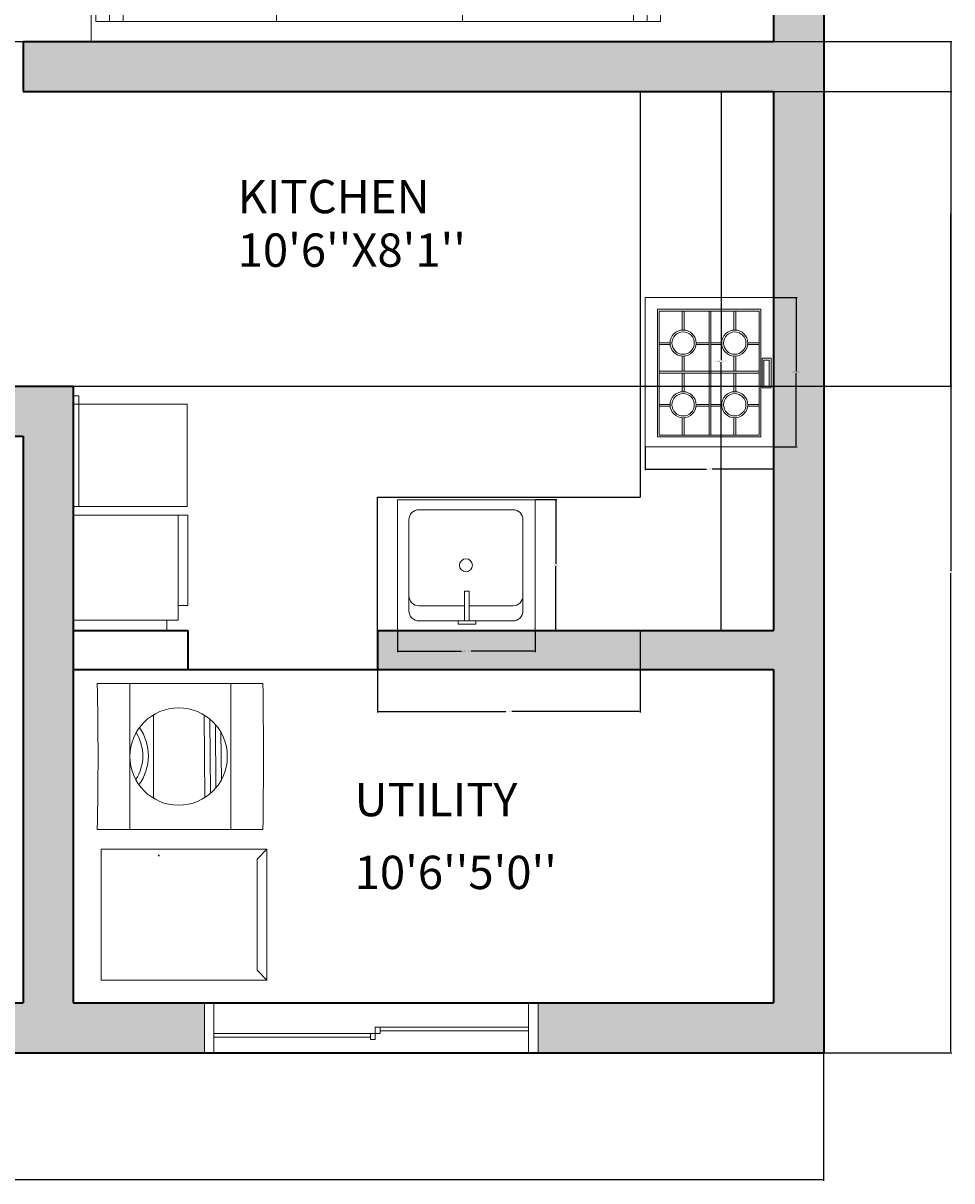
# Model space of a CAD drawing. Units: inches. Extents: x 1789 to 2841, y 3180 to 3702.
# Tile 4 of 14: x 2181 to 2348, y 3180 to 3388. Entities that reach past the tile are written whole.
import ezdxf

# ---------------------------------------------------------------- set-up
doc = ezdxf.new("R2010")
doc.units = ezdxf.units.IN
doc.header["$MEASUREMENT"] = 0
for name, color, linetype, lineweight in [('A-ANNO-DIMS', 2, 'Continuous', 18), ('A-AREA-IDEN', 7, 'Continuous', 18), ('A-EQPM', 8, 'Continuous', 18), ('A-FLOR-CASE', 34, 'Continuous', 25), ('A-FLOR-FIXT', 9, 'Continuous', 18), ('A-WALL', 40, 'Continuous', 35), ('A-WALL-PATT', 252, 'Continuous', 13), ('FURNITURE', 34, 'Continuous', 18), ('WINDOWS', 130, 'Continuous', 18)]:
    doc.layers.add(name, color=color, linetype=linetype, lineweight=lineweight)
doc.styles.get("Standard").update_dxf_attribs({"font": 'arial.ttf'})
doc.dimstyles.get("Standard").update_dxf_attribs({"dimtxt": 0.18, "dimasz": 0.18, "dimexe": 0.18, "dimexo": 0.0625, "dimgap": 0.09, "dimtad": 0, "dimtih": 1, "dimtoh": 1, "dimdec": 0, "dimzin": 0, "dimdsep": 46, "dimlunit": 3, "dimtxsty": 'Standard', "dimcen": 0.09, "dimadec": 0, "dimazin": 0, "dimtfac": 1, "dimtdec": 0, "dimtofl": 0, "dimtmove": 0, "dimatfit": 3, "dimfxl": 1, "dimtolj": 1, "dimtzin": 0, "dimarcsym": 0})

# ---------------------------------------------------------------- blocks, each defined once
blk = doc.blocks.new('HYJ')
for p, q in [((2236.02, 3650.77), (2262.74, 3650.77)), ((2236.02, 3650.11), (2262.74, 3650.11)), ((2206.12, 3649.67), (2234.3, 3649.67)), ((2206.12, 3649), (2234.3, 3649))]:
    blk.add_line(p, q)
for points in [[(2204.43, 3646.16), (2264.43, 3646.16), (2264.43, 3655.16), (2204.43, 3655.16)], [(2204.43, 3655.16), (2206.12, 3655.16), (2206.12, 3646.16), (2204.43, 3646.16)], [(2264.43, 3655.16), (2262.74, 3655.16), (2262.74, 3646.16), (2264.43, 3646.16)], [(2235.16, 3650.77), (2236.02, 3650.77), (2236.02, 3649.67), (2235.16, 3649.67)], [(2234.3, 3649.67), (2235.16, 3649.67), (2235.16, 3648.56), (2234.3, 3648.56)]]:
    blk.add_lwpolyline(points, close=True)
blk = doc.blocks.new('WASH')
for p, q in [((2194.57, 3269.63), (2224.37, 3269.63)), ((2200.44, 3243.35), (2200.44, 3269.63)), ((2218.58, 3269.63), (2218.58, 3243.35)), ((2204.7, 3264.01), (2204.68, 3248.99)), ((2213.79, 3263.95), (2213.93, 3249.12)), ((2214.8, 3263.23), (2214.92, 3249.86)), ((2215.81, 3262.24), (2215.91, 3250.86)), ((2216.82, 3260.81), (2216.9, 3252.31)), ((2194.57, 3243.35), (2224.37, 3243.35)), ((2225.07, 3239.8), (2223.31, 3238.03)), ((2223.31, 3218.04), (2223.31, 3238.03)), ((2225.07, 3216.27), (2223.31, 3218.04))]:
    blk.add_line(p, q)
blk.add_lwpolyline([(2195.28, 3239.8), (2225.07, 3239.8), (2225.07, 3216.27), (2195.28, 3216.27)], close=True)
blk.add_circle((2209.2, 3256.49), 8.76)
for centre, radius, start, end in [((1539.89, 3256.49), 654.81, 358.85012, 1.14988), ((1226.25, 3256.49), 998.2, 359.24572, 0.75428), ((2194.95, 3256.62), 7.81, 326.7676, 32.1994), ((2194.95, 3256.62), 8.81, 323.7828, 35.1842)]:
    blk.add_arc(centre, radius, start, end)
blk = doc.blocks.new('SINK')
for points in [[(2247.56, 3305.33), (2275.07, 3305.33), (2275.07, 3279.16), (2247.56, 3279.16)], [(2260.91, 3287.01), (2261.87, 3287.01), (2261.87, 3281.09), (2260.91, 3281.09)], [(2259.67, 3281.09), (2263.21, 3281.09), (2263.21, 3280.41), (2259.67, 3280.41)]]:
    blk.add_lwpolyline(points, close=True)
blk.add_lwpolyline([(2251.84, 3281.09), (2270.63, 3281.09, 0.414214), (2272.63, 3283.09), (2272.63, 3301.33, 0.414214), (2270.63, 3303.33), (2251.84, 3303.33, 0.414214), (2249.84, 3301.33), (2249.84, 3283.09, 0.414214)], format="xyb", close=True)
for points in [[(2249.84, 3301.33), (2249.84, 3286.11, 0.414214), (2251.84, 3284.11), (2260.91, 3284.11)], [(2261.87, 3284.11), (2270.63, 3284.11, 0.414214), (2272.63, 3286.11), (2272.63, 3301.33)]]:
    blk.add_lwpolyline(points, format="xyb")
blk.add_circle((2261.24, 3292.21), 1.3)
blk = doc.blocks.new('STOVE')
for p, q in [((2291.13, 3337.23), (2291.13, 3342.37)), ((2291.63, 3337.23), (2291.63, 3342.37)), ((2298.52, 3342.42), (2298.52, 3308.4)), ((2299.02, 3342.42), (2299.02, 3308.4)), ((2305.31, 3337.23), (2305.31, 3342.37)), ((2305.81, 3337.23), (2305.81, 3342.37)), ((2287.79, 3333.73), (2284.84, 3333.73)), ((2287.81, 3333.23), (2284.84, 3333.23)), ((2294.92, 3333.23), (2298.52, 3333.23)), ((2294.94, 3333.73), (2298.52, 3333.73)), ((2301.97, 3333.73), (2299.02, 3333.73)), ((2301.99, 3333.23), (2299.02, 3333.23)), ((2309.1, 3333.23), (2312.22, 3333.23)), ((2309.12, 3333.73), (2312.22, 3333.73)), ((2291.13, 3330.09), (2291.13, 3325.91)), ((2291.63, 3330.09), (2291.63, 3325.91)), ((2305.31, 3330.09), (2305.31, 3325.91)), ((2305.81, 3330.09), (2305.81, 3325.91)), ((2284.82, 3325.91), (2312.22, 3325.91)), ((2284.82, 3325.41), (2312.22, 3325.41)), ((2291.15, 3320.29), (2291.15, 3325.43)), ((2291.65, 3320.29), (2291.65, 3325.43)), ((2305.31, 3320.29), (2305.31, 3325.43)), ((2305.31, 3325.41), (2305.31, 3325.34)), ((2305.81, 3320.29), (2305.81, 3325.43)), ((2305.81, 3325.41), (2305.81, 3325.34)), ((2287.8, 3316.79), (2284.82, 3316.79)), ((2287.83, 3316.29), (2284.82, 3316.29)), ((2294.94, 3316.29), (2298.52, 3316.29)), ((2294.96, 3316.79), (2298.52, 3316.79)), ((2301.97, 3316.79), (2299.02, 3316.79)), ((2301.99, 3316.29), (2299.02, 3316.29)), ((2309.1, 3316.29), (2312.22, 3316.29)), ((2309.12, 3316.79), (2312.22, 3316.79)), ((2291.15, 3313.15), (2291.15, 3308.4)), ((2291.65, 3313.15), (2291.65, 3308.4)), ((2305.31, 3313.15), (2305.31, 3308.4)), ((2305.81, 3313.15), (2305.81, 3308.4))]:
    blk.add_line(p, q)
for points in [[(2280.96, 3346.14), (2316.23, 3346.14), (2316.23, 3305.13), (2280.96, 3305.13)], [(2284.32, 3342.92), (2312.72, 3342.92), (2312.72, 3307.9), (2284.32, 3307.9)], [(2284.82, 3342.42), (2312.22, 3342.42), (2312.22, 3308.4), (2284.82, 3308.4)], [(2313.05, 3329.49), (2315.55, 3329.49), (2315.55, 3321.33), (2313.05, 3321.33)], [(2313.55, 3328.99), (2315.05, 3328.99), (2315.05, 3321.83), (2313.55, 3321.83)]]:
    blk.add_lwpolyline(points, close=True)
for centre, radius in [((2291.37, 3333.66), 3.58), ((2291.37, 3333.66), 3.08), ((2305.55, 3333.66), 3.58), ((2305.55, 3333.66), 3.08), ((2291.38, 3316.72), 3.58), ((2291.38, 3316.72), 3.08), ((2305.55, 3316.72), 3.58), ((2305.55, 3316.72), 3.08)]:
    blk.add_circle(centre, radius)
blk = doc.blocks.new('BYY')
for p, q in [((2191.23, 3321.4), (2190.23, 3321.4)), ((2190.23, 3321.4), (2190.23, 3319.89)), ((2191.23, 3301.51), (2191.23, 3321.4)), ((2209.12, 3299.92), (2210.83, 3299.92)), ((2210.83, 3299.92), (2210.83, 3283.66)), ((2210.83, 3283.66), (2209.12, 3283.66)), ((2190.23, 3279.16), (2190.23, 3281.03)), ((2207.05, 3279.16), (2190.23, 3279.16)), ((2207.05, 3281.03), (2207.05, 3279.16))]:
    blk.add_line(p, q)
for points in [[(2190.23, 3319.89), (2210.75, 3319.89), (2210.75, 3301.51), (2190.23, 3301.51)], [(2190.23, 3281.03), (2209.12, 3281.03), (2209.12, 3299.92), (2190.23, 3299.92)]]:
    blk.add_lwpolyline(points, close=True)
blk = doc.blocks.new('SOFA')
for p, q in [((2185.57, 3479.13), (2185.57, 3482.99)), ((2185.57, 3482.99), (2290.09, 3482.99)), ((2290.09, 3482.99), (2290.09, 3460.33)), ((2159.93, 3439.46), (2194.03, 3439.46)), ((2226.79, 3388.76), (2226.79, 3418.07)), ((2260.29, 3388.76), (2260.29, 3418.07)), ((2310.14, 3409.22), (2310.14, 3394.77))]:
    blk.add_line(p, q)
for points in [[(2168.05, 3468.75), (2193.44, 3468.75), (2193.44, 3479.13), (2168.05, 3479.13)], [(2304.69, 3457.56), (2311.21, 3457.56), (2311.21, 3434.14), (2304.69, 3434.14)], [(2227.7, 3454.8), (2263.24, 3454.8), (2263.24, 3433.45), (2227.7, 3433.45)], [(2168.05, 3410.16), (2193.44, 3410.16), (2193.44, 3385.14), (2168.05, 3385.14)], [(2296.77, 3394.77), (2311.21, 3394.77), (2311.21, 3409.22), (2296.77, 3409.22)]]:
    blk.add_lwpolyline(points, close=True)
for points in [[(2168.05, 3467.86), (2168.05, 3470.06, 0.414214), (2166.05, 3472.06), (2155.57, 3472.06), (2155.57, 3406.2), (2166.05, 3406.2, 0.414214), (2168.05, 3408.2), (2168.05, 3411.06)], [(2308.49, 3457.56), (2308.49, 3460.33), (2286.26, 3460.33, 0.414214), (2285.26, 3459.33), (2285.26, 3455.79, 0.414214), (2286.26, 3454.79), (2304.69, 3454.79)], [(2308.49, 3434.14), (2308.49, 3431.37), (2286.26, 3431.37, -0.414214), (2285.26, 3432.37), (2285.26, 3435.9, -0.414214), (2286.26, 3436.9), (2304.69, 3436.9)], [(2196.77, 3407.83), (2196.77, 3416.07, -0.414214), (2198.77, 3418.07), (2291.47, 3418.07, -0.414214), (2293.47, 3416.07), (2293.47, 3407.83)], [(2293.47, 3393.66, 0.414214), (2291.47, 3395.66), (2198.77, 3395.66, 0.414214), (2196.77, 3393.66)]]:
    blk.add_lwpolyline(points, format="xyb")
for points in [[(2159.93, 3468.75), (2192.03, 3468.75, -0.414214), (2194.03, 3466.75), (2194.03, 3412.16, -0.414214), (2192.03, 3410.16), (2159.93, 3410.16)], [(2284.53, 3460.33), (2311.21, 3460.33), (2311.21, 3431.37), (2284.53, 3431.37, -0.414214), (2282.53, 3433.37), (2282.53, 3458.33, -0.414214)], [(2197.2, 3407.83), (2196.33, 3407.83, 0.414214), (2194.33, 3405.83), (2194.33, 3388.76), (2199.2, 3388.76), (2199.2, 3405.83, 0.414214)], [(2293.91, 3407.83), (2293.04, 3407.83, 0.414214), (2291.04, 3405.83), (2291.04, 3388.76), (2295.91, 3388.76), (2295.91, 3405.83, 0.414214)]]:
    blk.add_lwpolyline(points, format="xyb", close=True)
for points in [[(2168.05, 3455.52), (2168.05, 3459.94)], [(2168.05, 3429.95), (2168.05, 3448.97)], [(2168.05, 3423.4), (2168.05, 3422.93)], [(2168.05, 3418.98), (2168.05, 3422.93)], [(2293.47, 3393.66), (2293.47, 3388.76), (2196.77, 3388.76), (2196.77, 3393.66)], [(2196.77, 3388.76), (2293.47, 3388.76)]]:
    blk.add_lwpolyline(points)
for centre, radius in [((2265.18, 3410.2), 1.89), ((2303.99, 3401.99), 5.76)]:
    blk.add_circle(centre, radius)
for points, knots in [([(2162.46, 3458.3), (2163.29, 3460.04), (2164.26, 3462.07), (2164.89, 3465.65), (2164.78, 3467.36), (2164.69, 3468.75)], [0, 0, 0, 0, 5.733795, 6.696566, 10.854822, 10.854822, 10.854822, 10.854822]), ([(2164.69, 3468.75), (2166.38, 3468.37), (2168.87, 3467.8), (2171.7, 3465.95), (2173.26, 3465.49), (2174.05, 3465.25)], [0, 0, 0, 0, 5.14676, 7.56322, 10.027291, 10.027291, 10.027291, 10.027291]), ([(2174.05, 3465.25), (2173.89, 3464.58), (2173.37, 3462.38), (2172.69, 3460.22), (2172.22, 3458.71)], [0, 0, 0, 0, 2.055182, 6.796603, 6.796603, 6.796603, 6.796603]), ([(2162.46, 3458.3), (2163.64, 3458.13), (2165.71, 3457.83), (2167.35, 3456.54), (2168.05, 3455.99)], [0, 0, 0, 0, 3.512009, 6.140853, 6.140853, 6.140853, 6.140853]), ([(2168.05, 3459.94), (2169.55, 3459.7), (2172.38, 3459.25), (2174.06, 3456.94), (2174.85, 3455.84)], [0, 0, 0, 0, 4.35123, 8.24052, 8.24052, 8.24052, 8.24052]), ([(2173.18, 3446.97), (2173.68, 3448.57), (2174.42, 3450.93), (2174.65, 3453.95), (2174.79, 3455.29), (2174.85, 3455.84)], [0, 0, 0, 0, 5.016146, 7.373936, 9.056838, 9.056838, 9.056838, 9.056838]), ([(2166.66, 3449.86), (2167.7, 3449.17), (2169.71, 3447.85), (2172.05, 3447.25), (2173.18, 3446.97)], [0, 0, 0, 0, 3.710874, 7.178588, 7.178588, 7.178588, 7.178588]), ([(2166.66, 3429.05), (2167.7, 3429.74), (2169.71, 3431.07), (2172.05, 3431.66), (2173.18, 3431.95)], [0, 0, 0, 0, 3.710874, 7.178588, 7.178588, 7.178588, 7.178588]), ([(2173.18, 3431.95), (2173.68, 3430.35), (2174.42, 3427.99), (2174.65, 3424.97), (2174.79, 3423.63), (2174.85, 3423.07)], [0, 0, 0, 0, 5.016146, 7.373936, 9.056838, 9.056838, 9.056838, 9.056838]), ([(2162.46, 3420.62), (2163.64, 3420.79), (2165.71, 3421.09), (2167.35, 3422.37), (2168.05, 3422.93)], [0, 0, 0, 0, 3.512009, 6.140853, 6.140853, 6.140853, 6.140853]), ([(2168.05, 3418.98), (2169.55, 3419.22), (2172.38, 3419.66), (2174.06, 3421.98), (2174.85, 3423.07)], [0, 0, 0, 0, 4.35123, 8.24052, 8.24052, 8.24052, 8.24052]), ([(2162.46, 3420.62), (2163.29, 3418.88), (2164.26, 3416.85), (2164.89, 3413.27), (2164.78, 3411.56), (2164.69, 3410.16)], [0, 0, 0, 0, 5.733795, 6.696566, 10.854822, 10.854822, 10.854822, 10.854822]), ([(2174.05, 3413.67), (2173.89, 3414.33), (2173.37, 3416.54), (2172.69, 3418.7), (2172.22, 3420.21)], [0, 0, 0, 0, 2.055182, 6.796603, 6.796603, 6.796603, 6.796603]), ([(2164.69, 3410.16), (2166.38, 3410.55), (2168.87, 3411.12), (2171.7, 3412.96), (2173.26, 3413.43), (2174.05, 3413.67)], [0, 0, 0, 0, 5.14676, 7.56322, 10.027291, 10.027291, 10.027291, 10.027291])]:
    blk.add_open_spline(points, degree=3, knots=knots)
for points in [[(2168.05, 3455.52), (2167.85, 3453.6), (2167.25, 3451.73), (2166.66, 3449.86)], [(2168.05, 3423.4), (2167.85, 3425.31), (2167.25, 3427.18), (2166.66, 3429.05)]]:
    blk.add_open_spline(points, degree=3)
blk = doc.blocks.new('COUNTER-KITCHEN-L')
for p, q in [((47.28, 97), (47.28, 24)), ((0, 24), (47.28, 24)), ((0, 0), (0, 24))]:
    blk.add_line(p, q)
blk = doc.blocks.new('*D53')
at = {"layer": 'A-ANNO-DIMS', "color": 0, "lineweight": -2, "transparency": 16777216}
for p, q in [((2248.58, 3279.1), (2248.58, 3275.27)), ((2273.33, 3279.1), (2273.33, 3275.27)), ((2248.76, 3275.45), (2260.1, 3275.45)), ((2273.15, 3275.45), (2261.81, 3275.45))]:
    blk.add_line(p, q, dxfattribs=at)
at = {"layer": 'A-ANNO-DIMS', "color": 0, "transparency": 16777216}
for points in [[(2248.76, 3275.48), (2248.76, 3275.42), (2248.58, 3275.45)], [(2273.15, 3275.48), (2273.15, 3275.42), (2273.33, 3275.45)]]:
    blk.add_solid(points, dxfattribs=at)
at = {"layer": 'Defpoints', "color": 0, "transparency": 16777216}
for p in [(2248.58, 3279.16), (2273.33, 3279.16), (2273.33, 3275.45)]:
    blk.add_point(p, dxfattribs=at)
at = {"layer": 'A-ANNO-DIMS', "color": 0, "transparency": 16777216, "insert": (2260.96, 3275.45), "char_height": 0.18, "attachment_point": 5}
blk.add_mtext('\\A1;SINK 25 TYP.', dxfattribs=at)
blk = doc.blocks.new('*D54')
at = {"layer": 'A-ANNO-DIMS', "color": 0, "lineweight": -2, "transparency": 16777216}
for p, q in [((2273.4, 3302.71), (2277.23, 3302.71)), ((2277.05, 3302.53), (2277.05, 3291.11)), ((2277.05, 3279.34), (2277.05, 3290.75)), ((2273.4, 3279.16), (2277.23, 3279.16))]:
    blk.add_line(p, q, dxfattribs=at)
at = {"layer": 'A-ANNO-DIMS', "color": 0, "transparency": 16777216}
for points in [[(2277.02, 3302.53), (2277.08, 3302.53), (2277.05, 3302.71)], [(2277.02, 3279.34), (2277.08, 3279.34), (2277.05, 3279.16)]]:
    blk.add_solid(points, dxfattribs=at)
at = {"layer": 'Defpoints', "color": 0, "transparency": 16777216}
for p in [(2273.33, 3302.71), (2277.05, 3302.71), (2273.33, 3279.16)]:
    blk.add_point(p, dxfattribs=at)
at = {"layer": 'A-ANNO-DIMS', "color": 0, "transparency": 16777216, "insert": (2277.05, 3290.93), "char_height": 0.18, "attachment_point": 5}
blk.add_mtext('\\A1;24 TYP.', dxfattribs=at)
blk = doc.blocks.new('*D63')
at = {"layer": 'A-ANNO-DIMS', "color": 0, "lineweight": -2, "transparency": 16777216}
for p, q in [((2316.3, 3339.07), (2320.44, 3339.07)), ((2320.26, 3338.89), (2320.26, 3325.82)), ((2320.26, 3312.38), (2320.26, 3325.45)), ((2316.3, 3312.2), (2320.44, 3312.2))]:
    blk.add_line(p, q, dxfattribs=at)
at = {"layer": 'A-ANNO-DIMS', "color": 0, "transparency": 16777216}
for points in [[(2320.23, 3338.89), (2320.29, 3338.89), (2320.26, 3339.07)], [(2320.23, 3312.38), (2320.29, 3312.38), (2320.26, 3312.2)]]:
    blk.add_solid(points, dxfattribs=at)
at = {"layer": 'Defpoints', "color": 0, "transparency": 16777216}
for p in [(2316.23, 3339.07), (2320.26, 3339.07), (2316.23, 3312.2)]:
    blk.add_point(p, dxfattribs=at)
at = {"layer": 'A-ANNO-DIMS', "color": 0, "transparency": 16777216, "insert": (2320.26, 3325.64), "char_height": 0.18, "attachment_point": 5}
blk.add_mtext('\\A1;HOB 27 TYP.', dxfattribs=at)
blk = doc.blocks.new('*D64')
at = {"layer": 'A-ANNO-DIMS', "color": 0, "lineweight": -2, "transparency": 16777216}
for p, q in [((2293.12, 3312.14), (2293.12, 3307.99)), ((2316.23, 3312.14), (2316.23, 3307.99)), ((2293.3, 3308.17), (2304.15, 3308.17)), ((2316.05, 3308.17), (2305.2, 3308.17))]:
    blk.add_line(p, q, dxfattribs=at)
at = {"layer": 'A-ANNO-DIMS', "color": 0, "transparency": 16777216}
for points in [[(2293.3, 3308.2), (2293.3, 3308.14), (2293.12, 3308.17)], [(2316.05, 3308.2), (2316.05, 3308.14), (2316.23, 3308.17)]]:
    blk.add_solid(points, dxfattribs=at)
at = {"layer": 'Defpoints', "color": 0, "transparency": 16777216}
for p in [(2293.12, 3312.2), (2316.23, 3312.2), (2316.23, 3308.17)]:
    blk.add_point(p, dxfattribs=at)
at = {"layer": 'A-ANNO-DIMS', "color": 0, "transparency": 16777216, "insert": (2304.67, 3308.17), "char_height": 0.18, "attachment_point": 5}
blk.add_mtext('\\A1;23 TYP.', dxfattribs=at)
blk = doc.blocks.new('*D77')
at = {"layer": 'A-ANNO-DIMS', "color": 0, "lineweight": -2, "transparency": 16777216}
for p, q in [((2292.3, 3376.16), (2306.96, 3376.16)), ((2306.78, 3375.98), (2306.78, 3327.84)), ((2306.78, 3279.34), (2306.78, 3327.48)), ((2292.3, 3279.16), (2306.96, 3279.16))]:
    blk.add_line(p, q, dxfattribs=at)
at = {"layer": 'A-ANNO-DIMS', "color": 0, "transparency": 16777216}
for points in [[(2306.75, 3375.98), (2306.81, 3375.98), (2306.78, 3376.16)], [(2306.75, 3279.34), (2306.81, 3279.34), (2306.78, 3279.16)]]:
    blk.add_solid(points, dxfattribs=at)
at = {"layer": 'Defpoints', "color": 0, "transparency": 16777216}
for p in [(2292.23, 3376.16), (2306.78, 3376.16), (2292.23, 3279.16)]:
    blk.add_point(p, dxfattribs=at)
at = {"layer": 'A-ANNO-DIMS', "color": 0, "transparency": 16777216, "insert": (2306.78, 3327.66), "char_height": 0.18, "attachment_point": 5}
blk.add_mtext('\\A1;L-COUNTER 97 TYP.', dxfattribs=at)
blk = doc.blocks.new('*D78')
at = {"layer": 'A-ANNO-DIMS', "color": 0, "lineweight": -2, "transparency": 16777216}
for p, q in [((2244.95, 3279.1), (2244.95, 3264.43)), ((2292.23, 3279.1), (2292.23, 3264.43)), ((2245.13, 3264.61), (2268.06, 3264.61)), ((2292.05, 3264.61), (2269.12, 3264.61))]:
    blk.add_line(p, q, dxfattribs=at)
at = {"layer": 'A-ANNO-DIMS', "color": 0, "transparency": 16777216}
for points in [[(2245.13, 3264.64), (2245.13, 3264.58), (2244.95, 3264.61)], [(2292.05, 3264.64), (2292.05, 3264.58), (2292.23, 3264.61)]]:
    blk.add_solid(points, dxfattribs=at)
at = {"layer": 'Defpoints', "color": 0, "transparency": 16777216}
for p in [(2244.95, 3279.16), (2292.23, 3279.16), (2292.23, 3264.61)]:
    blk.add_point(p, dxfattribs=at)
at = {"layer": 'A-ANNO-DIMS', "color": 0, "transparency": 16777216, "insert": (2268.59, 3264.61), "char_height": 0.18, "attachment_point": 5}
blk.add_mtext('\\A1;47 TYP.', dxfattribs=at)
blk = doc.blocks.new('*D79')
at = {"layer": 'A-ANNO-DIMS', "color": 0, "lineweight": -2, "transparency": 16777216}
for p, q in [((1923.23, 3376.1), (1923.23, 3180.13)), ((2325.23, 3203.1), (2325.23, 3180.13)), ((1923.41, 3180.31), (2123.94, 3180.31)), ((2325.05, 3180.31), (2124.52, 3180.31))]:
    blk.add_line(p, q, dxfattribs=at)
at = {"layer": 'A-ANNO-DIMS', "color": 0, "transparency": 16777216}
for points in [[(1923.41, 3180.34), (1923.41, 3180.28), (1923.23, 3180.31)], [(2325.05, 3180.34), (2325.05, 3180.28), (2325.23, 3180.31)]]:
    blk.add_solid(points, dxfattribs=at)
at = {"layer": 'Defpoints', "color": 0, "transparency": 16777216}
for p in [(1923.23, 3376.16), (2325.23, 3203.16), (2325.23, 3180.31)]:
    blk.add_point(p, dxfattribs=at)
at = {"layer": 'A-ANNO-DIMS', "color": 0, "transparency": 16777216, "insert": (2124.23, 3180.31), "char_height": 0.18, "attachment_point": 5}
blk.add_mtext('\\A1;402', dxfattribs=at)
blk = doc.blocks.new('*D89')
at = {"layer": 'A-ANNO-DIMS', "color": 0, "lineweight": -2, "transparency": 16777216}
for p, q in [((2316.3, 3376.16), (2348.26, 3376.16)), ((2348.08, 3375.98), (2348.08, 3289.84)), ((2348.08, 3203.34), (2348.08, 3289.48)), ((2325.3, 3203.16), (2348.26, 3203.16))]:
    blk.add_line(p, q, dxfattribs=at)
at = {"layer": 'A-ANNO-DIMS', "color": 0, "transparency": 16777216}
for points in [[(2348.05, 3375.98), (2348.11, 3375.98), (2348.08, 3376.16)], [(2348.05, 3203.34), (2348.11, 3203.34), (2348.08, 3203.16)]]:
    blk.add_solid(points, dxfattribs=at)
at = {"layer": 'Defpoints', "color": 0, "transparency": 16777216}
for p in [(2316.23, 3376.16), (2325.23, 3203.16), (2348.08, 3203.16)]:
    blk.add_point(p, dxfattribs=at)
at = {"layer": 'A-ANNO-DIMS', "color": 0, "transparency": 16777216, "insert": (2348.08, 3289.66), "char_height": 0.18, "attachment_point": 5}
blk.add_mtext('\\A1;173', dxfattribs=at)
blk = doc.blocks.new('*D92')
at = {"layer": 'A-ANNO-DIMS', "color": 0, "lineweight": -2, "transparency": 16777216}
for p, q in [((2144.17, 3385.16), (2348.26, 3385.16)), ((2348.08, 3384.98), (2348.08, 3354.34)), ((2348.08, 3323.34), (2348.08, 3353.98)), ((2144.17, 3323.16), (2348.26, 3323.16))]:
    blk.add_line(p, q, dxfattribs=at)
at = {"layer": 'A-ANNO-DIMS', "color": 0, "transparency": 16777216}
for points in [[(2348.05, 3384.98), (2348.11, 3384.98), (2348.08, 3385.16)], [(2348.05, 3323.34), (2348.11, 3323.34), (2348.08, 3323.16)]]:
    blk.add_solid(points, dxfattribs=at)
at = {"layer": 'Defpoints', "color": 0, "transparency": 16777216}
for p in [(2144.11, 3385.16), (2348.08, 3385.16), (2144.11, 3323.16)]:
    blk.add_point(p, dxfattribs=at)
at = {"layer": 'A-ANNO-DIMS', "color": 0, "transparency": 16777216, "insert": (2348.08, 3354.16), "char_height": 0.18, "attachment_point": 5}
blk.add_mtext('\\A1;62', dxfattribs=at)
blk = doc.blocks.new('*D116')
at = {"layer": 'A-ANNO-DIMS', "color": 0, "lineweight": -2, "transparency": 16777216}
for p, q in [((1789.65, 3701.85), (1789.83, 3701.85)), ((1789.83, 3701.85), (1945.65, 3528.3)), ((2205.56, 3238.68), (2205.74, 3238.68)), ((2205.65, 3238.59), (2205.65, 3238.77))]:
    blk.add_line(p, q, dxfattribs=at)
at = {"layer": 'A-ANNO-DIMS', "color": 0, "transparency": 16777216}
blk.add_solid([(1945.67, 3528.32), (1945.62, 3528.28), (1945.77, 3528.16)], dxfattribs=at)
at = {"layer": 'Defpoints', "color": 0, "transparency": 16777216}
for p in [(1945.77, 3528.16), (2205.65, 3238.68)]:
    blk.add_point(p, dxfattribs=at)
at = {"layer": 'A-ANNO-DIMS', "color": 0, "transparency": 16777216, "insert": (1789.28, 3701.85), "char_height": 0.18, "attachment_point": 5}
blk.add_mtext('\\A1;R389', dxfattribs=at)

msp = doc.modelspace()

# ---------------------------------------------------------------- hatches: boundary and pattern name
at = {"layer": 'A-WALL-PATT'}
h = msp.add_hatch(color=256, dxfattribs=at)
h.dxf.hatch_style = 1
h.paths.add_polyline_path([(2316.2333, 3385.1608), (2193.4449, 3385.1608), (2193.4449, 3385.1441), (2181.2333, 3385.1441), (2181.2333, 3376.1608), (2316.2333, 3376.1608), (2316.2333, 3279.1608), (2244.9532, 3279.1608), (2244.9532, 3272.1608), (2316.2333, 3272.1608), (2316.2333, 3212.1608), (2273.8514, 3212.1608), (2273.8514, 3203.1608), (2325.2333, 3203.1608), (2325.2333, 3473.1608), (2319.2333, 3473.1608, -0.01876983), (2316.2333, 3473.2734)])
h = msp.add_hatch(color=256, dxfattribs=at)
h.dxf.hatch_style = 1
h.paths.add_polyline_path([(2213.8514, 3203.1608), (2213.8514, 3212.1608), (2190.2333, 3212.1608), (2190.2333, 3323.1608), (2121.2333, 3323.1608), (2121.2333, 3385.1608), (2107.924, 3385.1608), (2107.924, 3379.1608), (2107.924, 3376.1608), (2112.2333, 3376.1608), (2112.2333, 3269.2132), (2118.2333, 3269.2132), (2121.2333, 3269.2132), (2121.2333, 3314.1608), (2181.2333, 3314.1608), (2181.2333, 3212.1608), (2178.3707, 3212.1608), (2178.3707, 3203.1608)])
h.paths.add_polyline_path([(2050.2092, 3264.3521), (2108.2631, 3264.3521), (2108.2631, 3273.6652), (2050.2092, 3273.6652)], flags=9)

# ---------------------------------------------------------------- linework, layer by layer
at = {"layer": 'A-WALL'}
for p, q in [((2316.2333, 3473.2734), (2316.2333, 3385.1608)), ((2325.2333, 3473.1608), (2325.2333, 3203.1608)), ((2181.2333, 3385.1608), (2181.2333, 3376.1608)), ((2181.2333, 3385.1608), (2316.2333, 3385.1608)), ((2181.2333, 3376.1608), (2316.2333, 3376.1608)), ((2316.2333, 3376.1608), (2316.2333, 3279.1608)), ((2121.2333, 3323.1608), (2190.2333, 3323.1608)), ((2190.2333, 3323.1608), (2190.2333, 3212.1608)), ((2121.2333, 3314.1608), (2181.2333, 3314.1608)), ((2181.2333, 3314.1608), (2181.2333, 3212.1608)), ((2190.2333, 3279.1608), (2210.8305, 3279.1608)), ((2210.8305, 3279.1608), (2210.8305, 3272.1608)), ((2244.9532, 3279.1608), (2244.9532, 3272.1608)), ((2244.9532, 3279.1608), (2316.2333, 3279.1608)), ((2190.2333, 3272.1608), (2316.2333, 3272.1608)), ((2316.2333, 3272.1608), (2316.2333, 3212.1608)), ((2121.2333, 3212.1608), (2181.2333, 3212.1608)), ((2190.2333, 3212.1608), (2316.2333, 3212.1608)), ((1959.2333, 3203.1608), (2325.2333, 3203.1608))]:
    msp.add_line(p, q, dxfattribs=at)

# ---------------------------------------------------------------- block references
at = {"layer": 'A-EQPM', "xscale": 0.6553007250005952, "yscale": 0.6553007250005952, "zscale": 0.6553007250005952}
msp.add_blockref('STOVE', (798.404, 1146.3444), dxfattribs=at)
at = {"layer": 'A-EQPM'}
for name in ['BYY', 'WASH']:
    msp.add_blockref(name, (0, 0), dxfattribs=at)
at = {"layer": 'A-FLOR-CASE'}
msp.add_blockref('COUNTER-KITCHEN-L', (2244.953, 3279.161), dxfattribs=at)
at = {"layer": 'A-FLOR-FIXT', "xscale": 0.8998033160254596, "yscale": 0.8998033160254596, "zscale": 0.8998033160254596}
msp.add_blockref('SINK', (226.22, 328.561), dxfattribs=at)
at = {"layer": 'FURNITURE'}
msp.add_blockref('SOFA', (0, 0), dxfattribs=at)
at = {"layer": 'WINDOWS'}
msp.add_blockref('HYJ', (9.4189, -443), dxfattribs=at)

# ---------------------------------------------------------------- texts
at = {"layer": 'A-ANNO-DIMS'}
for s, p in [("10'6''X8'1''", (2219.8164, 3344.6141)), ("10'6''5'0''", (2240.8634, 3232.6388))]:
    msp.add_text(s, height=6, dxfattribs=at).set_placement(p)
at = {"layer": 'A-AREA-IDEN'}
for s, p in [('KITCHEN', (2219.8164, 3354.2526)), ('UTILITY', (2240.8634, 3245.7371))]:
    msp.add_text(s, height=6, dxfattribs=at).set_placement(p)

# ---------------------------------------------------------------- dimensions: what is measured, and where the dimension line sits
at = {"layer": 'A-ANNO-DIMS'}
dim = msp.add_radius_dim(center=(2205.6545, 3238.6823), mpoint=(1945.766, 3528.162), dimstyle='Standard', override={"dimdec": 0, "dimlfac": 1, "dimrnd": 0, "dimzin": 0, "dimdsep": 46, "dimlunit": 2}, dxfattribs=at)
dim.commit()
dim.dimension.update_dxf_attribs({"geometry": '*D116', "text_midpoint": (1789.2778, 3701.8498), "dimtype": 164})
for base, p1, p2, picture, middle in [((2348.0833, 3385.1608), (2144.1086, 3323.1608), (2144.1086, 3385.1608), '*D92', (2348.0833, 3354.1608)), ((2348.0833, 3203.1608), (2316.2333, 3376.1608), (2325.2333, 3203.1608), '*D89', (2348.0833, 3289.6608))]:
    dim = msp.add_linear_dim(base=base, p1=p1, p2=p2, angle=90, dimstyle='Standard', override={"dimdec": 0, "dimlfac": 1, "dimrnd": 0, "dimzin": 0, "dimdsep": 46, "dimlunit": 2}, dxfattribs=at)
    dim.commit()
    dim.dimension.update_dxf_attribs({"geometry": picture, "text_midpoint": middle})
dim = msp.add_linear_dim(base=(2325.2333, 3180.3108), p1=(1923.2333, 3376.1608), p2=(2325.2333, 3203.1608), dimstyle='Standard', override={"dimdec": 0, "dimlfac": 1, "dimrnd": 0, "dimzin": 0, "dimdsep": 46, "dimlunit": 2}, dxfattribs=at)
dim.commit()
dim.dimension.update_dxf_attribs({"geometry": '*D79', "text_midpoint": (2124.2333, 3180.3108)})
for base, p1, p2, text, picture, middle in [((2306.7833, 3376.1608), (2292.2333, 3279.1608), (2292.2333, 3376.1608), 'L-COUNTER <> TYP.', '*D77', (2306.7833, 3327.6608)), ((2320.2645, 3339.0734), (2316.2333, 3312.1992), (2316.2333, 3339.0734), 'HOB <> TYP.', '*D63', (2320.2645, 3325.6363)), ((2277.048, 3302.7057), (2273.3348, 3279.1608), (2273.3348, 3302.7057), '<> TYP.', '*D54', (2277.048, 3290.9332))]:
    dim = msp.add_linear_dim(base=base, p1=p1, p2=p2, angle=90, text=text, dimstyle='Standard', override={"dimdec": 0, "dimlfac": 1, "dimrnd": 0, "dimzin": 0, "dimdsep": 46, "dimlunit": 2}, dxfattribs=at)
    dim.commit()
    dim.dimension.update_dxf_attribs({"geometry": picture, "text_midpoint": middle})
for base, p1, p2, text, picture, middle in [((2316.2333, 3308.1681), (2293.1166, 3312.1992), (2316.2333, 3312.1992), '<> TYP.', '*D64', (2304.675, 3308.1681)), ((2292.2333, 3264.6108), (2244.9532, 3279.1608), (2292.2333, 3279.1608), '<> TYP.', '*D78', (2268.5933, 3264.6108)), ((2273.3348, 3275.4476), (2248.58, 3279.1608), (2273.3348, 3279.1608), 'SINK <> TYP.', '*D53', (2260.9574, 3275.4476))]:
    dim = msp.add_linear_dim(base=base, p1=p1, p2=p2, text=text, dimstyle='Standard', override={"dimdec": 0, "dimlfac": 1, "dimrnd": 0, "dimzin": 0, "dimdsep": 46, "dimlunit": 2}, dxfattribs=at)
    dim.commit()
    dim.dimension.update_dxf_attribs({"geometry": picture, "text_midpoint": middle})

doc.saveas('drawing.dxf')
